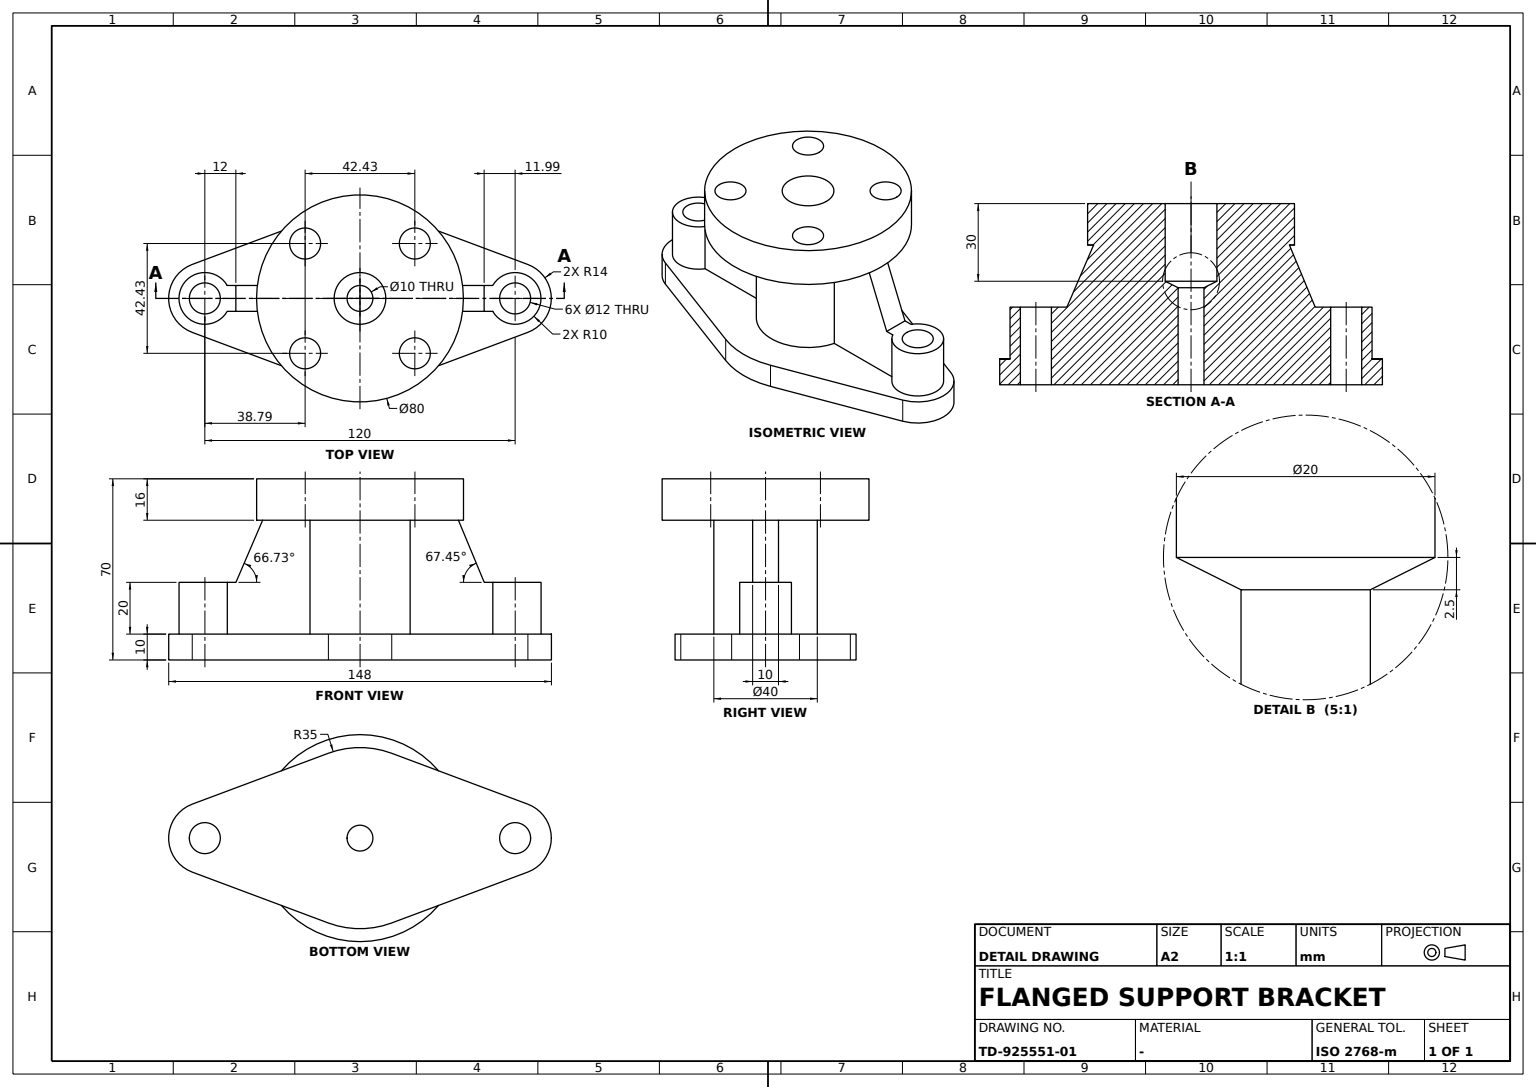
CATIA V5 part; units mm, degrees
ref_plane "Plane1" through (0, 0, 100) normal (0, 0, 1) x (1, 0, 0)
sketch "Sketch1" plane through (0, 0, 0) normal (0, 0, 1) x (1, 0, 0)
  arc A0 (-12.25, -32.7862) -> (12.25, -32.7862) centre (0, 0) ccw
  arc A1 (64.9, -13.1145) -> (64.9, 13.1145) centre (60, 0) ccw
  point P0 (60, 0)
  arc A2 (-64.9, 13.1145) -> (-64.9, -13.1145) centre (-60, 0) ccw
  point P1 (-60, 0)
  line L0 (-64.9, 13.1145) -> (-12.25, 32.7862)
  line L1 (-64.9, -13.1145) -> (-12.25, -32.7862)
  line L2 (12.25, 32.7862) -> (64.9, 13.1145)
  point P2 (12.25, 32.7862)
  line L3 (12.25, -32.7862) -> (64.9, -13.1145)
  arc A3 (12.25, 32.7862) -> (-12.25, 32.7862) centre (0, 0) ccw
  dimension "radius A0" = 35
  dimension "radius A1" = 14
  dimension "distance P0 y axis" = 60
  dimension "radius A2" = 14
  dimension "distance P1 y axis" = 60
  constraint coincidence P0 x-axis
  constraint coincidence P1 x-axis
  constraint coincidence P2 A0
  constraint coincidence A0 A3
  constraint tangency L0 A2
  constraint tangency L0 A0
  constraint tangency L1 A2
  constraint tangency L1 A0
  constraint tangency L2 A0
  constraint tangency L2 A1
  constraint tangency L3 A1
  constraint tangency L3 A0
extrude "Pad1" add sketch "Sketch1" along normal blind 10
sketch "Sketch2" plane through (0, 0, 10) normal (0, 0, 1) x (1, 0, 0)
  circle A0 centre (0, 0) radius 20
  dimension "radius A0" = 20
extrude "Pad2" add sketch "Sketch2" along normal blind 44
sketch "Sketch3" plane through (0, 0, 54) normal (0, 0, 1) x (1, 0, 0)
  circle A0 centre (0, 0) radius 40
  arc A1 (12.25, 32.7862) -> (-12.25, 32.7862) centre (0, 0) ccw construction
  dimension "radius A0" = 40
  constraint concentricity A0 A1
extrude "Pad3" add sketch "Sketch3" along normal blind 16
sketch "Sketch4" plane through (0, 0, 70) normal (0, 0, 1) x (1, 0, 0)
  circle A0 centre (0, 0) radius 30 construction
  circle A1 centre (0, 0) radius 40 construction
  line L0 (0, 0) -> (54.8742, 54.8742) construction
  circle A2 centre (21.2132, 21.2132) radius 6
  point P0 (21.2132, 21.2132)
  line L1 (0, 0) -> (-45.6097, -45.6097) construction
  circle A3 centre (-21.2132, -21.2132) radius 6
  point P1 (-21.2132, -21.2132)
  point P2 (-16.5676, -25.0103)
  circle A4 centre (-21.2132, 21.2132) radius 6
  circle A5 centre (21.2132, -21.2132) radius 6
  dimension "radius A0" = 30
  dimension "angle L0 x axis" = 45
  dimension "radius A2" = 6
  dimension "angle L1 x axis" = 45
  dimension "radius A3" = 6
  constraint concentricity A0 A1
  constraint coincidence P0 L0
  constraint coincidence P0 A0
  constraint coincidence P1 L1
  constraint coincidence P1 A0
  constraint coincidence A3 P2
  constraint coincidence P2 A0
  constraint symmetry A2 A4 y-axis
  constraint symmetry A3 A5 y-axis
extrude "Pocket1" cut sketch "Sketch4" against normal blind 16
sketch "Sketch5" plane through (0, 0, 10) normal (0, 0, 1) x (1, 0, 0)
  circle A0 centre (60, 0) radius 10
  arc A1 (64.9, -13.1145) -> (64.9, 13.1145) centre (60, 0) ccw construction
  circle A2 centre (-60, 0) radius 10
  arc A3 (-64.9, 13.1145) -> (-64.9, -13.1145) centre (-60, 0) ccw construction
  dimension "radius A0" = 10
  dimension "radius A2" = 10
  constraint concentricity A0 A1
  constraint concentricity A2 A3
extrude "Pad4" add sketch "Sketch5" along normal blind 20
sketch "Sketch6" plane through (0, 0, 30) normal (0, 0, 1) x (1, 0, 0)
  circle A0 centre (60, 0) radius 6
  circle A1 centre (60, 0) radius 10 construction
  dimension "radius A0" = 6
  constraint concentricity A0 A1
extrude "Pocket2" cut sketch "Sketch6" against normal through all
sketch "Sketch7" plane through (0, 0, 30) normal (0, 0, 1) x (1, 0, 0)
  circle A0 centre (-60, 0) radius 6
  circle A1 centre (-60, 0) radius 10 construction
  dimension "radius A0" = 6
  constraint concentricity A0 A1
extrude "Pocket3" cut sketch "Sketch7" against normal through all
sketch "Sketch8" plane through (0, 0, 70) normal (0, 0, 1) x (1, 0, 0)
  point P0 (0, 0)
hole "Hole1" at (0, 0, 70) direction (0, 0, -1) diameter 20 depth 30
sketch "Sketch9" plane through (0, 0, 40) normal (0, 0, 1) x (1, 0, 0)
  point P0 (0, 0)
hole "Hole2" at (0, 0, 40) direction (0, 0, -1) diameter 10 depth 40
sketch "Sketch10" plane through (0, 0, 0) normal (0, 1, 0) x (-1, 0, 0)
  line L0 (10, 40) -> (5, 37.5)
  point P0 (0, 35)
  point P1 (10, 40)
  line L1 (5, 40) -> (-5, 40) construction
  line L2 (10, 40) -> (5, 40)
  point P2 (10, 40)
  line L3 (5, 40) -> (5, 37.5)
  dimension "distance P0 L1" = 5
  dimension "distance P1 y axis" = 10
  dimension "distance P1 P0 y axis" = 5
  dimension "distance L3 y axis" = 5
  constraint coincidence P0 y-axis
  constraint coincidence P2 L0
  constraint coincidence P2 P1
  constraint horizontal L2 x-axis
  constraint vertical L3 y-axis
revolve "Groove1" cut sketch "Sketch10" angle 360 about axis through (0, 0, 0) along (0, 0, 1)
sketch "Sketch11" plane through (0, 0, 0) normal (0, 1, 0) x (-1, 0, 0)
  line L0 (-50.277, 30) -> (-48.0116, 30)
  point P0 (-50.277, 30)
  line L1 (-70, 30) -> (-50, 30) construction
  line L2 (-48.0116, 30) -> (-37.9745, 54.168)
  constraint horizontal L0 x-axis
  constraint coincidence P0 L1
rib "Stiffener1" sketch "Sketch11" thickness 10 sides both
sketch "Sketch12" plane through (0, 0, 0) normal (0, 1, 0) x (-1, 0, 0)
  line L0 (50.5392, 30) -> (48, 30)
  point P0 (48, 30)
  line L1 (50, 30) -> (70, 30) construction
  line L2 (48, 30) -> (37.5316, 54.3384)
  dimension "D1" = 12
  constraint horizontal L0 x-axis
  constraint coincidence L0 L1
rib "Stiffener2" sketch "Sketch12" thickness 10 sides both
